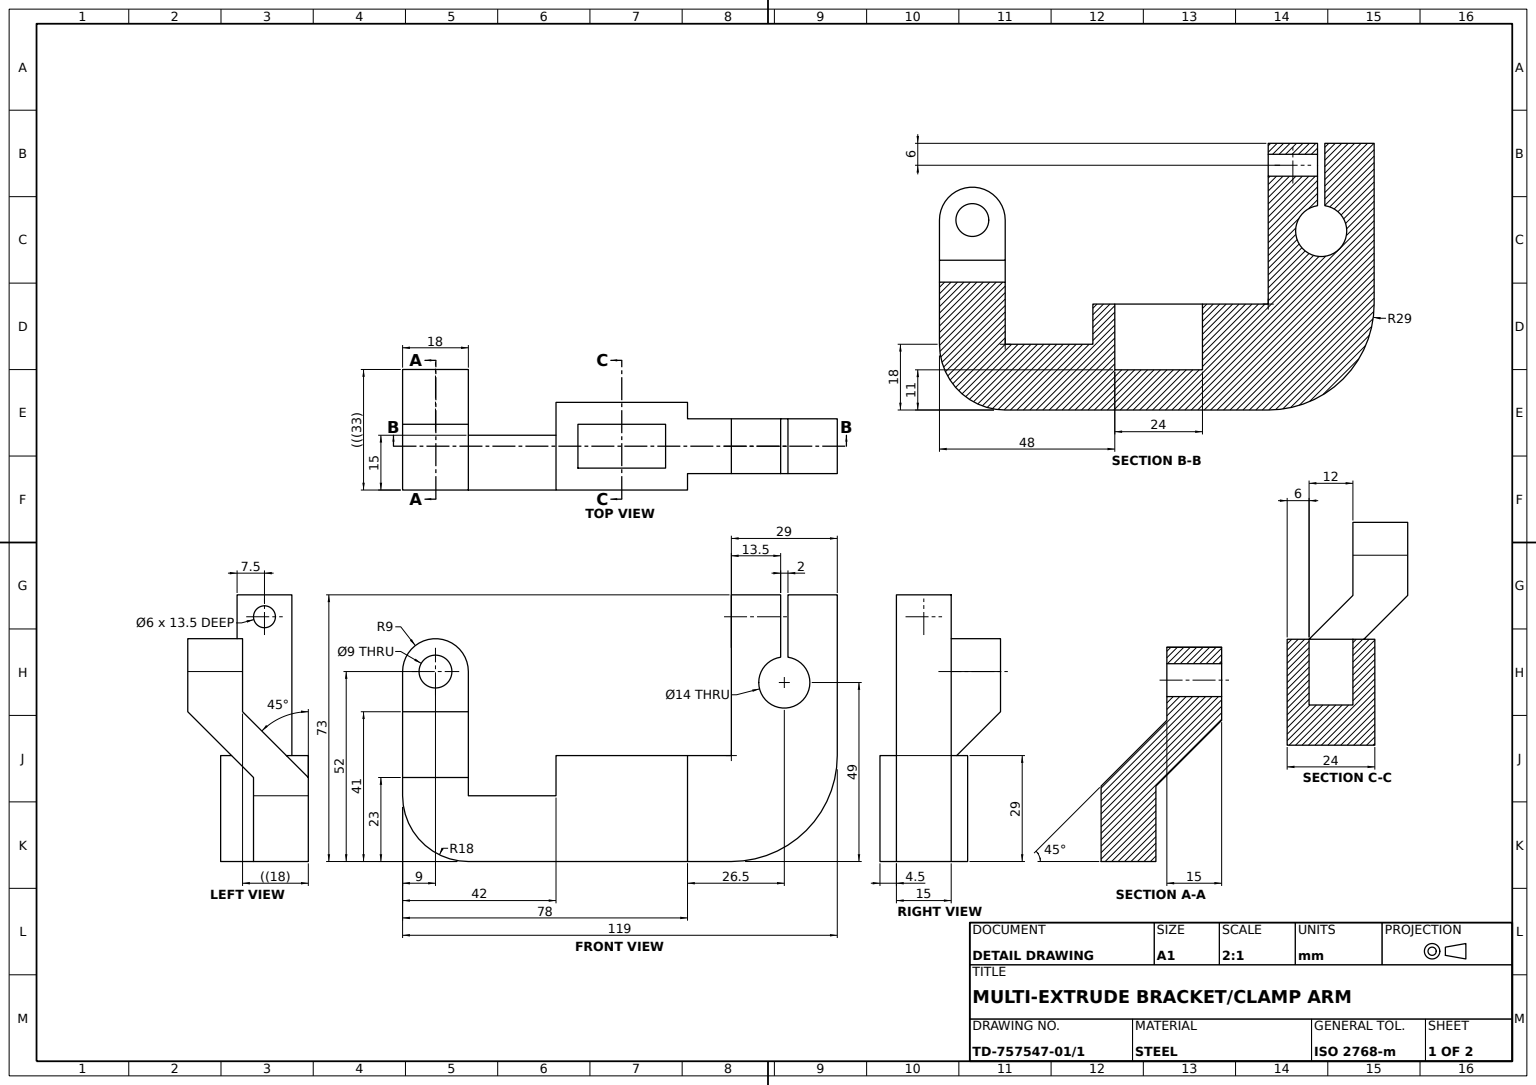
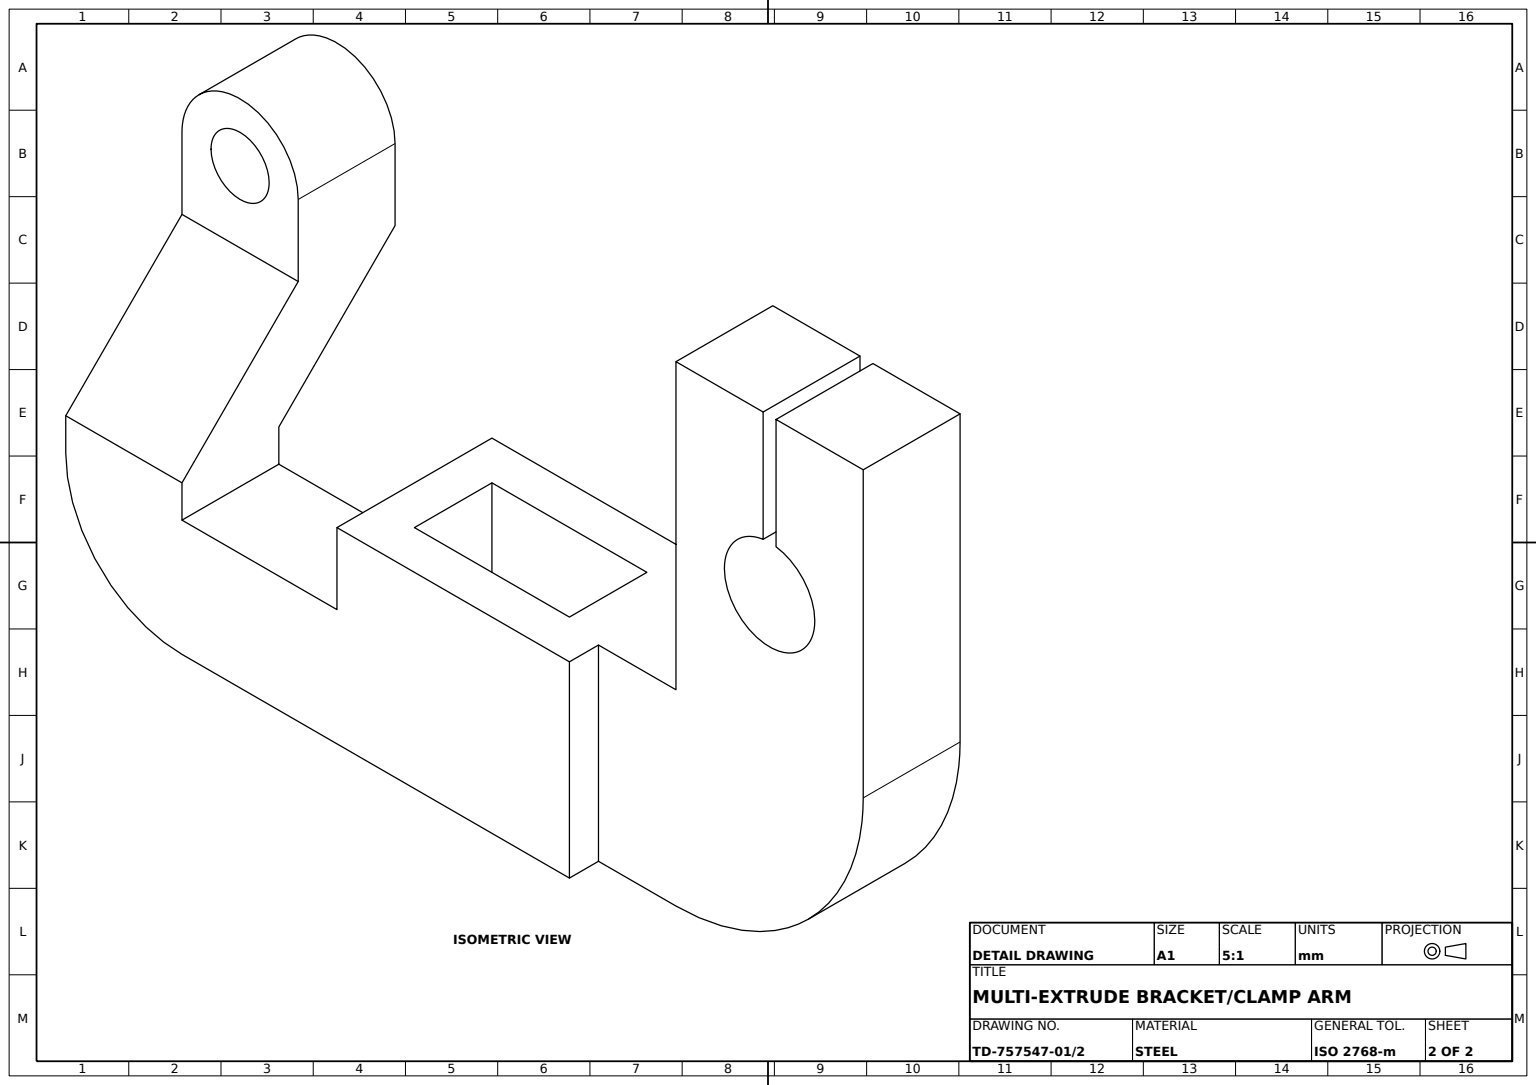
from build123d import *

# Parameters (mm, degrees)
BASE_BODY_DEPTH             = 15
ARM_BLOCK_DEPTH             = 18
INCLINED_ARM_SKETCH_W       = 15
INCLINED_ARM_SKETCH_H       = 11
INCLINED_ARM_DEPTH          = 18
TOP_LUG_DEPTH               = 15
LUG_HOLE_SKETCH_R           = 4.5
LUG_HOLE_9_DEPTH            = 15
POCKET_BOSS_SKETCH_W        = 36
POCKET_BOSS_SKETCH_H        = 29
POCKET_BOSS_DEPTH           = 9
CLEVIS_BLOCK_SKETCH_W       = 12
CLEVIS_BLOCK_SKETCH_H       = 15
CLEVIS_BLOCK_DEPTH          = 29
CLEVIS_CORNER_DEPTH         = 15
CLEVIS_JAW_DEPTH            = 15
CLEVIS_HOLE_SKETCH_R        = 7
CLEVIS_HOLE_14_DEPTH        = 15
CLEVIS_SLOT_DEPTH           = 18
JAW_HOLE_SKETCH_R           = 3
JAW_HOLE_6_DEPTH            = 15
RECTANGULAR_POCKET_SKETCH_W = 24
RECTANGULAR_POCKET_SKETCH_H = 12
RECTANGULAR_POCKET_DEPTH    = 18


with BuildPart() as part:
    # Base Profile Sketch → Base Body (new body)
    with BuildSketch(Plane.XY):
        with BuildLine():
            Line((0, -18), (60, -18))
            Line((60, -18), (60, 11))
            Line((60, 11), (24, 11))
            Line((24, 11), (24, 0))
            Line((24, 0), (0, 0))
            Line((0, 0), (0, 5))
            Line((0, 5), (-18, 5))
            Line((-18, 5), (-18, 0))
            ThreePointArc((-18, 0), (-12.727922061, -12.727922061), (0, -18))
        make_face()
    extrude(amount=BASE_BODY_DEPTH)

    # Arm Block Sketch → Arm Block (add)
    with BuildSketch(Plane.ZY.offset(18)):
        Polygon((-18, 23), (-3, 23), (15, 5), (0, 5), align=None)
    extrude(amount=-ARM_BLOCK_DEPTH)

    # Inclined Arm Sketch → Inclined Arm (add)
    with BuildSketch(Plane.ZY.offset(18)):
        with Locations((-10.5, 28.5)):
            Rectangle(INCLINED_ARM_SKETCH_W, INCLINED_ARM_SKETCH_H)
    extrude(amount=-INCLINED_ARM_DEPTH)

    # Top Lug Sketch → Top Lug (add)
    with BuildSketch(Plane.XY.offset(-3)):
        with BuildLine():
            Line((-18, 34), (0, 34))
            ThreePointArc((0, 34), (-9, 43), (-18, 34))
        make_face()
    extrude(amount=-TOP_LUG_DEPTH)

    # Lug Hole Sketch → Lug Hole Ø9 (cut)
    with BuildSketch(Plane.XY.offset(-3)):
        with Locations((-9, 34)):
            Circle(LUG_HOLE_SKETCH_R)
    extrude(amount=-LUG_HOLE_9_DEPTH, mode=Mode.SUBTRACT)

    # Pocket Boss Sketch → Pocket Boss (add)
    with BuildSketch(Plane(origin=(0, 0, 0), x_dir=(-1, 0, 0), z_dir=(0, 0, -1))):
        with Locations((-42, -3.5)):
            Rectangle(POCKET_BOSS_SKETCH_W, POCKET_BOSS_SKETCH_H)
    extrude(amount=POCKET_BOSS_DEPTH)

    # Clevis Block Sketch → Clevis Block (add)
    with BuildSketch(Plane(origin=(0, 11, 0), x_dir=(1, 0, 0), z_dir=(0, 1, 0))):
        with Locations((66, -3)):
            Rectangle(CLEVIS_BLOCK_SKETCH_W, CLEVIS_BLOCK_SKETCH_H)
    extrude(amount=-CLEVIS_BLOCK_DEPTH)

    # Clevis Corner Sketch → Clevis Corner (add)
    with BuildSketch(Plane.XY.offset(10.5)):
        with BuildLine():
            Line((72, 11), (101, 11))
            ThreePointArc((101, 11), (92.506096654, -9.506096654), (72, -18))
            Line((72, -18), (72, 11))
        make_face()
    extrude(amount=-CLEVIS_CORNER_DEPTH)

    # Clevis Jaw Sketch → Clevis Jaw (add)
    with BuildSketch(Plane.XY.offset(10.5)):
        Polygon((101, 11), (72, 11), (72, 31), (72, 55), (101, 55), align=None)
    extrude(amount=-CLEVIS_JAW_DEPTH)

    # Clevis Hole Sketch → Clevis Hole Ø14 (cut)
    with BuildSketch(Plane.XY.offset(10.5)):
        with Locations((86.5, 31)):
            Circle(CLEVIS_HOLE_SKETCH_R)
    extrude(amount=-CLEVIS_HOLE_14_DEPTH, mode=Mode.SUBTRACT)

    # Clevis Slot Sketch → Clevis Slot (cut)
    with BuildSketch(Plane(origin=(0, 55, 0), x_dir=(1, 0, 0), z_dir=(0, 1, 0))):
        Polygon((86.5, 4.5), (85.5, 4.5), (85.5, -10.5), (87.5, -10.5), (87.5, 4.5), align=None)
    extrude(amount=-CLEVIS_SLOT_DEPTH, mode=Mode.SUBTRACT)

    # Jaw Hole Sketch → Jaw Hole Ø6 (cut)
    with BuildSketch(Plane.ZY.offset(-72)):
        with Locations((3, 49)):
            Circle(JAW_HOLE_SKETCH_R)
    extrude(amount=-JAW_HOLE_6_DEPTH, mode=Mode.SUBTRACT)

    # Rectangular Pocket Sketch → Rectangular Pocket (cut)
    with BuildSketch(Plane(origin=(0, 11, 0), x_dir=(1, 0, 0), z_dir=(0, 1, 0))):
        with Locations((42, -3)):
            Rectangle(RECTANGULAR_POCKET_SKETCH_W, RECTANGULAR_POCKET_SKETCH_H)
    extrude(amount=-RECTANGULAR_POCKET_DEPTH, mode=Mode.SUBTRACT)


solid = part.part
